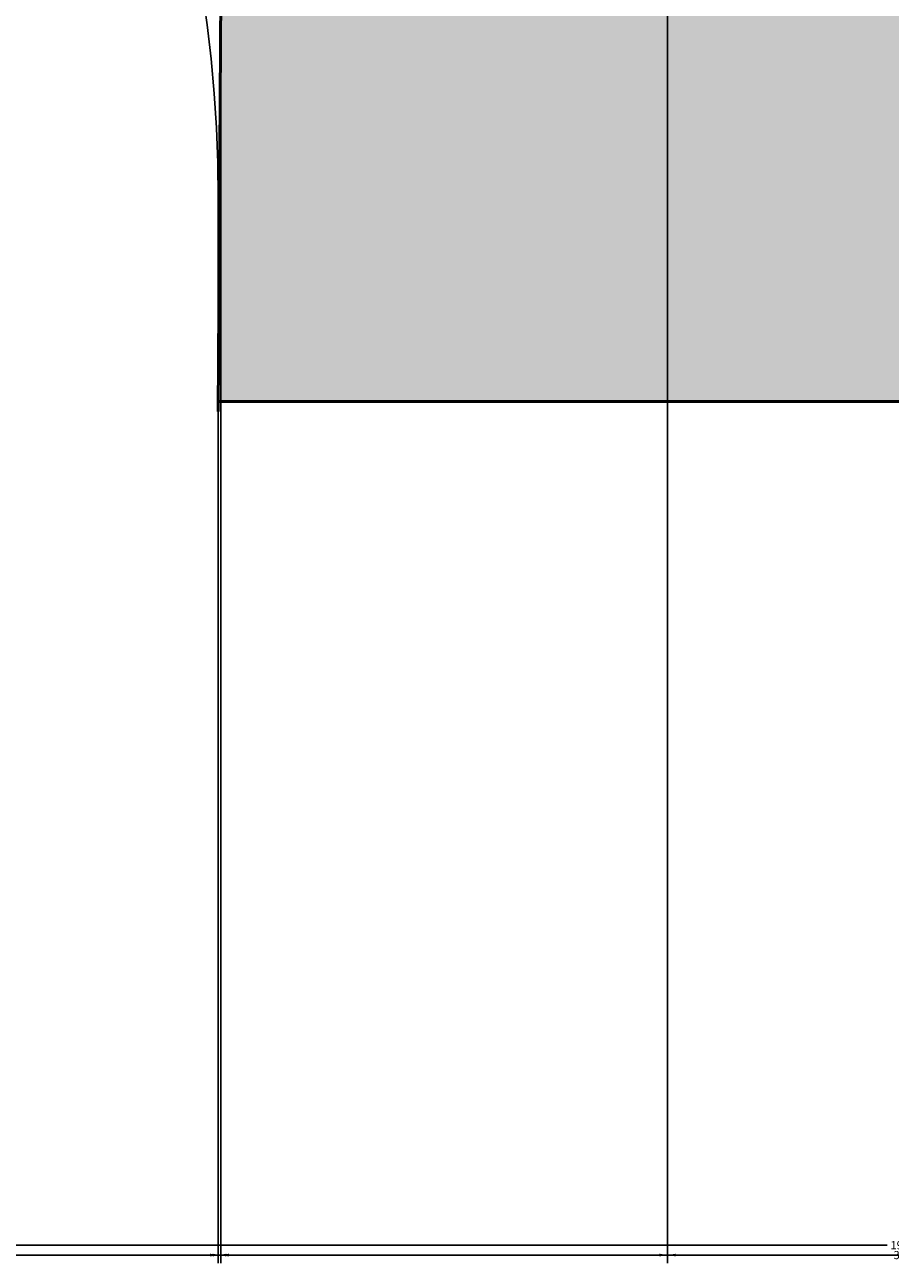
# Model space of a CAD drawing. Units: inches. Extents: x 2231 to 2461, y 2045 to 2455.
# Tile 13 of 95: x 2326 to 2346, y 2045 to 2072. Entities that reach past the tile are written whole.
import ezdxf

# ---------------------------------------------------------------- set-up
doc = ezdxf.new("R2010")
doc.units = ezdxf.units.IN
for name, color, linetype, lineweight in [('A-ANNO-DIMS', 2, 'Continuous', 18), ('A-DOOR', 3, 'Continuous', 25), ('A-WALL', 7, 'Continuous', 50)]:
    doc.layers.add(name, color=color, linetype=linetype, lineweight=lineweight)
doc.layers.add('A-WALL-PATT', color=18, linetype='Continuous', lineweight=13, true_color=0x000000)
doc.styles.get("Standard").update_dxf_attribs({"font": 'arial.ttf'})
doc.dimstyles.get("Standard").update_dxf_attribs({"dimtxt": 0.18, "dimasz": 0.18, "dimexe": 0.18, "dimexo": 0.0625, "dimgap": 0.09, "dimtad": 0, "dimtih": 1, "dimtoh": 1, "dimdec": 4, "dimzin": 0, "dimdsep": 46, "dimtxsty": 'Standard', "dimcen": 0.09, "dimadec": 0, "dimazin": 0, "dimtfac": 1, "dimtdec": 4, "dimtofl": 0, "dimtmove": 0, "dimatfit": 3, "dimfxl": 1, "dimtolj": 1, "dimtzin": 0, "dimarcsym": 0})

# ---------------------------------------------------------------- blocks, each defined once
blk = doc.blocks.new('*U5')
blk.add_line((40, 0), (40, -6))
blk.add_arc((0, 0), 40, 0, 90)
blk = doc.blocks.new('*D33')
at = {"layer": 'A-ANNO-DIMS', "color": 0, "lineweight": -2, "transparency": 16777216}
for p, q in [((2249.794, 2063.77), (2249.794, 2045.02)), ((2441.794, 2063.77), (2441.794, 2045.02)), ((2249.974, 2045.2), (2345.514, 2045.2)), ((2441.614, 2045.2), (2346.073, 2045.2))]:
    blk.add_line(p, q, dxfattribs=at)
at = {"layer": 'A-ANNO-DIMS', "color": 0, "transparency": 16777216}
for points in [[(2249.974, 2045.23), (2249.974, 2045.17), (2249.794, 2045.2)], [(2441.614, 2045.23), (2441.614, 2045.17), (2441.794, 2045.2)]]:
    blk.add_solid(points, dxfattribs=at)
at = {"layer": 'Defpoints', "color": 0, "transparency": 16777216}
for p in [(2249.794, 2063.833), (2441.794, 2063.833), (2249.794, 2045.2)]:
    blk.add_point(p, dxfattribs=at)
at = {"layer": 'A-ANNO-DIMS', "color": 0, "transparency": 16777216, "insert": (2345.794, 2045.2), "char_height": 0.18, "attachment_point": 5}
blk.add_mtext('\\A1;192', dxfattribs=at)
blk = doc.blocks.new('*D45')
at = {"layer": 'A-ANNO-DIMS', "color": 0, "lineweight": -2, "transparency": 16777216}
for p, q in [((2300.739, 2063.77), (2300.739, 2044.803)), ((2330.74, 2063.77), (2330.74, 2044.803)), ((2300.919, 2044.983), (2315.521, 2044.983)), ((2330.56, 2044.983), (2315.958, 2044.983))]:
    blk.add_line(p, q, dxfattribs=at)
at = {"layer": 'A-ANNO-DIMS', "color": 0, "transparency": 16777216}
for points in [[(2300.919, 2045.013), (2300.919, 2044.953), (2300.739, 2044.983)], [(2330.56, 2045.013), (2330.56, 2044.953), (2330.74, 2044.983)]]:
    blk.add_solid(points, dxfattribs=at)
at = {"layer": 'Defpoints', "color": 0, "transparency": 16777216}
for p in [(2300.739, 2063.833), (2330.74, 2063.833), (2330.74, 2044.983)]:
    blk.add_point(p, dxfattribs=at)
at = {"layer": 'A-ANNO-DIMS', "color": 0, "transparency": 16777216, "insert": (2315.739, 2044.983), "char_height": 0.18, "attachment_point": 5}
blk.add_mtext('\\A1;30', dxfattribs=at)
blk = doc.blocks.new('*D46')
at = {"layer": 'A-ANNO-DIMS', "color": 0, "lineweight": -2, "transparency": 16777216}
for p, q in [((2330.74, 2063.77), (2330.74, 2044.803)), ((2368.664, 2063.77), (2368.664, 2044.803)), ((2330.92, 2044.983), (2349.239, 2044.983)), ((2368.484, 2044.983), (2350.165, 2044.983))]:
    blk.add_line(p, q, dxfattribs=at)
at = {"layer": 'A-ANNO-DIMS', "color": 0, "transparency": 16777216}
for points in [[(2330.92, 2045.013), (2330.92, 2044.953), (2330.74, 2044.983)], [(2368.484, 2045.013), (2368.484, 2044.953), (2368.664, 2044.983)]]:
    blk.add_solid(points, dxfattribs=at)
at = {"layer": 'Defpoints', "color": 0, "transparency": 16777216}
for p in [(2330.74, 2063.833), (2368.664, 2063.833), (2368.664, 2044.983)]:
    blk.add_point(p, dxfattribs=at)
at = {"layer": 'A-ANNO-DIMS', "color": 0, "transparency": 16777216, "insert": (2349.702, 2044.983), "char_height": 0.18, "attachment_point": 5}
blk.add_mtext('\\A1;37.924', dxfattribs=at)
blk = doc.blocks.new('*D51')
at = {"layer": 'A-ANNO-DIMS', "color": 0, "lineweight": -2, "transparency": 16777216}
for p, q in [((2258.794, 2306.77), (2258.794, 2044.803)), ((2330.794, 2306.77), (2330.794, 2044.803)), ((2258.974, 2044.983), (2294.576, 2044.983)), ((2330.614, 2044.983), (2295.011, 2044.983))]:
    blk.add_line(p, q, dxfattribs=at)
at = {"layer": 'A-ANNO-DIMS', "color": 0, "transparency": 16777216}
for points in [[(2258.974, 2045.013), (2258.974, 2044.953), (2258.794, 2044.983)], [(2330.614, 2045.013), (2330.614, 2044.953), (2330.794, 2044.983)]]:
    blk.add_solid(points, dxfattribs=at)
at = {"layer": 'Defpoints', "color": 0, "transparency": 16777216}
for p in [(2258.794, 2306.833), (2330.794, 2306.833), (2330.794, 2044.983)]:
    blk.add_point(p, dxfattribs=at)
at = {"layer": 'A-ANNO-DIMS', "color": 0, "transparency": 16777216, "insert": (2294.794, 2044.983), "char_height": 0.18, "attachment_point": 5}
blk.add_mtext('\\A1;72', dxfattribs=at)
blk = doc.blocks.new('*D52')
at = {"layer": 'A-ANNO-DIMS', "color": 0, "lineweight": -2, "transparency": 16777216}
for p, q in [((2330.794, 2306.77), (2330.794, 2044.803)), ((2360.794, 2306.77), (2360.794, 2044.803)), ((2330.974, 2044.983), (2345.575, 2044.983)), ((2360.614, 2044.983), (2346.012, 2044.983))]:
    blk.add_line(p, q, dxfattribs=at)
at = {"layer": 'A-ANNO-DIMS', "color": 0, "transparency": 16777216}
for points in [[(2330.974, 2045.013), (2330.974, 2044.953), (2330.794, 2044.983)], [(2360.614, 2045.013), (2360.614, 2044.953), (2360.794, 2044.983)]]:
    blk.add_solid(points, dxfattribs=at)
at = {"layer": 'Defpoints', "color": 0, "transparency": 16777216}
for p in [(2330.794, 2306.833), (2360.794, 2306.833), (2360.794, 2044.983)]:
    blk.add_point(p, dxfattribs=at)
at = {"layer": 'A-ANNO-DIMS', "color": 0, "transparency": 16777216, "insert": (2345.794, 2044.983), "char_height": 0.18, "attachment_point": 5}
blk.add_mtext('\\A1;30', dxfattribs=at)
blk = doc.blocks.new('*D65')
at = {"layer": 'A-ANNO-DIMS', "color": 0, "lineweight": -2, "transparency": 16777216}
for p, q in [((2285.635, 2189.285), (2285.635, 2044.803)), ((2340.667, 2189.285), (2340.667, 2044.803)), ((2285.815, 2044.983), (2312.758, 2044.983)), ((2340.487, 2044.983), (2313.545, 2044.983))]:
    blk.add_line(p, q, dxfattribs=at)
at = {"layer": 'A-ANNO-DIMS', "color": 0, "transparency": 16777216}
for points in [[(2285.815, 2045.013), (2285.815, 2044.953), (2285.635, 2044.983)], [(2340.487, 2045.013), (2340.487, 2044.953), (2340.667, 2044.983)]]:
    blk.add_solid(points, dxfattribs=at)
at = {"layer": 'Defpoints', "color": 0, "transparency": 16777216}
for p in [(2285.635, 2189.348), (2340.667, 2189.348), (2340.667, 2044.983)]:
    blk.add_point(p, dxfattribs=at)
at = {"layer": 'A-ANNO-DIMS', "color": 0, "transparency": 16777216, "insert": (2313.151, 2044.983), "char_height": 0.18, "attachment_point": 5}
blk.add_mtext('\\A1;55.03', dxfattribs=at)
blk = doc.blocks.new('*D69')
at = {"layer": 'A-ANNO-DIMS', "color": 0, "lineweight": -2, "transparency": 16777216}
for p, q in [((2340.667, 2189.285), (2340.667, 2044.803)), ((2394.794, 2186.77), (2394.794, 2044.803)), ((2340.847, 2044.983), (2367.337, 2044.983)), ((2394.614, 2044.983), (2368.124, 2044.983))]:
    blk.add_line(p, q, dxfattribs=at)
at = {"layer": 'A-ANNO-DIMS', "color": 0, "transparency": 16777216}
for points in [[(2340.847, 2045.013), (2340.847, 2044.953), (2340.667, 2044.983)], [(2394.614, 2045.013), (2394.614, 2044.953), (2394.794, 2044.983)]]:
    blk.add_solid(points, dxfattribs=at)
at = {"layer": 'Defpoints', "color": 0, "transparency": 16777216}
for p in [(2340.667, 2189.348), (2394.794, 2186.833), (2394.794, 2044.983)]:
    blk.add_point(p, dxfattribs=at)
at = {"layer": 'A-ANNO-DIMS', "color": 0, "transparency": 16777216, "insert": (2367.73, 2044.983), "char_height": 0.18, "attachment_point": 5}
blk.add_mtext('\\A1;54.13', dxfattribs=at)

msp = doc.modelspace()

# ---------------------------------------------------------------- hatches: boundary and pattern name
at = {"layer": 'A-WALL-PATT'}
h = msp.add_hatch(color=256, dxfattribs=at)
h.dxf.hatch_style = 1
h.paths.add_polyline_path([(2441.7935, 2269.1535), (2432.7935, 2269.1535), (2432.7935, 2186.8328), (2396.7935, 2186.8328), (2396.7935, 2286.8328), (2394.7935, 2286.8328), (2394.7935, 2186.8328), (2334.7935, 2186.8328), (2334.7935, 2182.8328), (2432.7935, 2182.8328), (2432.7935, 2072.8328), (2416.6639, 2072.8328), (2416.6639, 2063.8328), (2441.7935, 2063.8328)])
h.paths.add_polyline_path([(2368.6639, 2072.8328), (2367.04, 2072.8328), (2330.7942, 2072.8328), (2330.7397, 2063.8328), (2368.6639, 2063.8328)])
h.paths.add_polyline_path([(2300.7392, 2068.3328), (2300.7392, 2072.8328), (2298.7935, 2072.8328), (2294.7935, 2072.8328), (2258.7935, 2072.8328), (2258.7935, 2120.8328), (2294.7935, 2120.8328), (2298.7935, 2120.8328), (2298.7935, 2128.8328), (2294.7935, 2128.8328), (2294.7935, 2124.8328), (2258.7935, 2124.8328), (2258.7935, 2182.8328), (2294.7935, 2182.8328), (2294.7935, 2174.8328), (2298.7935, 2174.8328), (2298.7935, 2182.8328), (2304.7935, 2182.8328), (2304.7935, 2186.8328), (2258.7935, 2186.8328), (2258.7935, 2221.999), (2249.7935, 2221.999), (2249.7935, 2063.8328), (2300.7392, 2063.8328)])
h.paths.add_polyline_path([(2391.9338, 2435.8328), (2333.82, 2435.8328), (2333.82, 2426.8328), (2368.7935, 2426.8328), (2368.7935, 2374.9508), (2368.7935, 2370.8328), (2372.3935, 2370.8328), (2372.7935, 2370.8328), (2372.7935, 2426.8328), (2391.9338, 2426.8328)])
h.paths.add_polyline_path([(2441.7935, 2435.8328), (2415.9338, 2435.8328), (2415.9338, 2426.8328), (2432.7935, 2426.8328), (2432.7935, 2334.8328), (2372.7935, 2334.8328), (2372.7935, 2346.8328), (2368.7935, 2346.8328), (2368.7935, 2306.8328), (2360.7935, 2306.8328), (2360.7935, 2302.8328), (2368.7935, 2302.8328), (2372.7935, 2302.8328), (2372.7935, 2330.8328), (2432.7935, 2330.8328), (2432.7935, 2317.1535), (2441.7935, 2317.1535)])
h.paths.add_polyline_path([(2285.82, 2435.8328), (2249.7935, 2435.8328), (2249.7935, 2269.999), (2258.7935, 2269.999), (2258.7935, 2302.8328), (2318.8168, 2302.8328), (2330.7935, 2302.8328), (2330.7935, 2306.8328), (2258.7935, 2306.8328), (2258.7935, 2426.8328), (2285.82, 2426.8328)])

# ---------------------------------------------------------------- linework, layer by layer
at = {"layer": 'A-WALL'}
msp.add_line((2330.7942, 2072.8328), (2330.7384, 2063.615), dxfattribs=at)
msp.add_lwpolyline([(2300.7392, 2063.8328), (2249.7935, 2063.8328), (2249.7935, 2435.8328), (2441.7935, 2435.8328), (2441.7935, 2063.8328), (2330.7397, 2063.8328)], dxfattribs=at)

# ---------------------------------------------------------------- block references
at = {"layer": 'A-DOOR', "xscale": 0.75, "yscale": 0.75, "zscale": 0.75}
msp.add_blockref('*U5', (2300.7392, 2068.3328), dxfattribs=at)

# ---------------------------------------------------------------- dimensions: what is measured, and where the dimension line sits
at = {"layer": 'A-ANNO-DIMS'}
for base, p1, p2, override, picture, middle in [((2330.7935, 2044.9825), (2258.7935, 2306.8328), (2330.7935, 2306.8328), {"dimdec": 0, "dimlfac": 1, "dimrnd": 0, "dimzin": 0, "dimdsep": 46, "dimlunit": 2}, '*D51', (2294.7935, 2044.9825)), ((2360.7935, 2044.9825), (2330.7935, 2306.8328), (2360.7935, 2306.8328), {"dimdec": 0, "dimlfac": 1, "dimrnd": 0, "dimzin": 0, "dimdsep": 46, "dimlunit": 2}, '*D52', (2345.7935, 2044.9825)), ((2340.6673, 2044.9825), (2285.6353, 2189.3477), (2340.6673, 2189.3477), {"dimdec": 2, "dimlfac": 1, "dimrnd": 0, "dimzin": 0, "dimdsep": 46, "dimlunit": 2}, '*D65', (2313.1513, 2044.9825)), ((2394.7935, 2044.9825), (2340.6673, 2189.3477), (2394.7935, 2186.8328), {"dimdec": 2, "dimlfac": 1, "dimrnd": 0, "dimzin": 0, "dimdsep": 46, "dimlunit": 2}, '*D69', (2367.7304, 2044.9825)), ((2330.7397, 2044.9825), (2300.7392, 2063.8328), (2330.7397, 2063.8328), {"dimdec": 0, "dimlfac": 1, "dimrnd": 0, "dimzin": 0, "dimdsep": 46, "dimlunit": 2}, '*D45', (2315.7395, 2044.9825)), ((2368.6639, 2044.9825), (2330.7397, 2063.8328), (2368.6639, 2063.8328), {"dimdec": 3, "dimlfac": 1, "dimrnd": 0, "dimzin": 0, "dimdsep": 46, "dimlunit": 2}, '*D46', (2349.7018, 2044.9825))]:
    dim = msp.add_linear_dim(base=base, p1=p1, p2=p2, dimstyle='Standard', override=override, dxfattribs=at)
    dim.commit()
    dim.dimension.update_dxf_attribs({"geometry": picture, "text_midpoint": middle})
dim = msp.add_linear_dim(base=(2249.7935, 2045.2003), p1=(2441.7935, 2063.8328), p2=(2249.7935, 2063.8328), angle=180, dimstyle='Standard', override={"dimdec": 0, "dimlfac": 1, "dimrnd": 0, "dimzin": 0, "dimdsep": 46, "dimlunit": 2}, dxfattribs=at)
dim.commit()
dim.dimension.update_dxf_attribs({"geometry": '*D33', "text_midpoint": (2345.7935, 2045.2003)})

doc.saveas('drawing.dxf')
